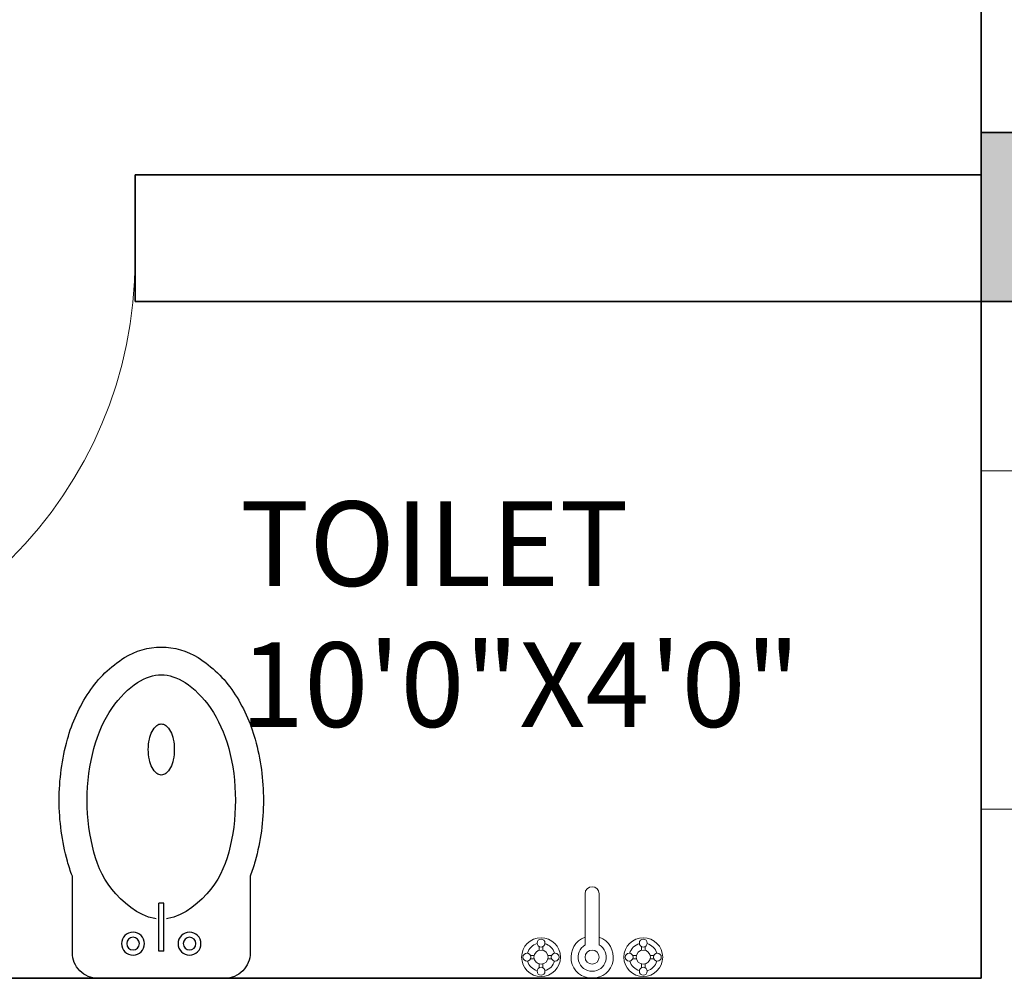
# Model space of a CAD drawing. Units: inches. Extents: x 3321 to 5237, y 11 to 1752.
# Tile 10 of 43: x 3724 to 3793, y 1377 to 1445. Entities that reach past the tile are written whole.
import ezdxf

# ---------------------------------------------------------------- set-up
doc = ezdxf.new("R2010")
doc.units = ezdxf.units.IN
for name, color, linetype, lineweight in [('A-ANNO-DIMS', 2, 'Continuous', 18), ('A-AREA-IDEN', 7, 'Continuous', 18), ('A-COLS', 1, 'Continuous', 35), ('A-DOOR', 4, 'Continuous', 18), ('A-GLAZ', 5, 'Continuous', 18), ('A-WALL', 7, 'Continuous', 35), ('Сантехника', 7, 'Continuous', 18)]:
    doc.layers.add(name, color=color, linetype=linetype, lineweight=lineweight)
doc.layers.add('SANTEH', color=7, linetype='Continuous')
doc.styles.get("Standard").update_dxf_attribs({"font": 'arial.ttf'})
doc.dimstyles.new('ISO-25', dxfattribs={"dimtxt": 9, "dimasz": 2.5, "dimexe": 1.25, "dimexo": 0.625, "dimtad": 1, "dimdec": 1, "dimlunit": 3, "dimtxsty": 'Standard', "dimcen": 2.5, "dimclrd": 4, "dimclre": 4, "dimclrt": 256, "dimadec": 0, "dimazin": 0, "dimtfac": 1, "dimtdec": 1, "dimtmove": 0, "dimatfit": 3, "dimfxl": 1, "dimarcsym": 0})

# ---------------------------------------------------------------- blocks, each defined once
blk = doc.blocks.new('*U5')
for p, q in [((0, 0), (0, -6)), ((-30, 0), (-30, -6))]:
    blk.add_line(p, q)
blk.add_lwpolyline([(0, 0), (0, 30), (-1.75, 30), (-1.75, 0)], close=True)
blk.add_arc((0, 0), 30, 90, 180)
blk = doc.blocks.new('K10-45')
at = {"layer": 'SANTEH'}
for p, q in [((-18.9, 83.4), (-18.9, 177.1)), ((-18.9, 177.1), (-8.9, 177.1)), ((-8.9, 83.4), (-8.9, 177.1)), ((-18.9, 83.4), (-8.9, 83.4))]:
    blk.add_line(p, q, dxfattribs=at)
for points in [[(160.3, 230.4, 0.023928), (169.9, 259.6, 0.067459), (186.1, 379, 0.067459), (169.9, 498.4, 0.079812), (127.5, 591.1, 0.107118), (58, 658.5, 0.139889), (-13.9, 679, 0.139889), (-85.8, 658.5, 0.107118), (-155.3, 591.1, 0.079812), (-197.7, 498.4, 0.067459), (-213.9, 379, 0.067459), (-197.7, 259.6, 0.023928), (-188.1, 230.4), (-188.1, 80.2, 0.414214), (-138.1, 30.2), (110.3, 30.2, 0.414214), (160.3, 80.2)], [(-39.4, 478.5, 0.052061), (-37.3, 458.3, 0.065919), (-32, 443.1, 0.104629), (-22.6, 431.5, 0.172287), (-13.9, 428.4, 0.172287), (-5.2, 431.5, 0.104629), (4.1, 443.1, 0.065919), (9.5, 458.3, 0.052061), (11.6, 478.5, 0.052061), (9.5, 498.7, 0.065919), (4.1, 513.9, 0.104629), (-5.2, 525.5, 0.172287), (-13.9, 528.6, 0.172287), (-22.6, 525.5, 0.104629), (-32, 513.9, 0.065919), (-37.3, 498.7, 0.052061)]]:
    blk.add_lwpolyline(points, format="xyb", close=True, dxfattribs=at)
blk.add_lwpolyline([(-3.9, 147), (-1.4, 147.2), (10.9, 150.3), (23, 155.1), (34.7, 161.4), (45.9, 168.8), (56.5, 177.2), (66.3, 186.2), (75.2, 195.5), (83.2, 205), (90.3, 214.7), (96.5, 224.5), (102, 234.5), (106.9, 244.7), (111.1, 255.3), (114.8, 266.2), (118.1, 277.6), (121.1, 289.3), (123.7, 301.4), (126, 313.8), (127.9, 326.5), (129.3, 339.5), (130.4, 352.6), (131.1, 365.8), (131.3, 379), (131.1, 392.2), (130.4, 405.4), (129.3, 418.5), (127.9, 431.4), (126, 444.2), (123.7, 456.6), (121.1, 468.7), (118.1, 480.4), (114.8, 491.7), (111.2, 502.6), (107.3, 513.1), (103, 523.1), (98.4, 532.7), (93.5, 541.9), (88.3, 550.7), (82.8, 559.1), (77.1, 567.1), (71, 574.6), (64.9, 581.7), (58.5, 588.3), (52.1, 594.4), (45.7, 600), (39.3, 605), (33, 609.4), (26.9, 613.2), (20.8, 616.4), (14.9, 619), (9, 621.1), (3.2, 622.7), (-2.5, 623.8), (-8.2, 624.5), (-13.9, 624.7), (-19.6, 624.5), (-25.3, 623.8), (-31, 622.7), (-36.8, 621.1), (-42.7, 619), (-48.6, 616.4), (-54.7, 613.2), (-60.9, 609.4), (-67.2, 605), (-73.5, 600), (-80, 594.4), (-86.4, 588.3), (-92.7, 581.7), (-98.9, 574.6), (-104.9, 567.1), (-110.6, 559.1), (-116.1, 550.7), (-121.3, 541.9), (-126.2, 532.7), (-130.8, 523.1), (-135.1, 513.1), (-139, 502.6), (-142.7, 491.7), (-146, 480.4), (-148.9, 468.7), (-151.5, 456.6), (-153.8, 444.2), (-155.7, 431.4), (-157.2, 418.5), (-158.2, 405.4), (-158.9, 392.2), (-159.1, 379), (-158.9, 365.8), (-158.2, 352.6), (-157.2, 339.5), (-155.7, 326.5), (-153.8, 313.8), (-151.5, 301.4), (-148.9, 289.3), (-146, 277.6), (-142.6, 266.2), (-138.9, 255.3), (-134.7, 244.7), (-129.8, 234.5), (-124.4, 224.5), (-118.1, 214.7), (-111, 205), (-103.1, 195.5), (-94.1, 186.2), (-84.3, 177.2), (-73.7, 168.8), (-62.5, 161.4), (-50.8, 155.1), (-38.7, 150.3), (-26.4, 147.2), (-23.9, 147)], dxfattribs=at)
for centre, radius in [((-69.2, 98.1), 22.4), ((41.4, 98.1), 22.4), ((-69.2, 98.1), 12.4), ((41.4, 98.1), 12.4)]:
    blk.add_circle(centre, radius, dxfattribs=at)
blk = doc.blocks.new('Faucet - Bathroom top')
for p, q in [((-3.75, 0.4788), (-3.75, 0.75)), ((-3.5, 0.482), (-3.5, 0.75)), ((3.5, 0.4788), (3.5, 0.75)), ((3.75, 0.482), (3.75, 0.75)), ((-4.107, 0.125), (-4.375, 0.125)), ((-3.1461, 0.125), (-2.875, 0.125)), ((3.143, 0.125), (2.875, 0.125)), ((4.1039, 0.125), (4.375, 0.125)), ((-4.1039, -0.125), (-4.375, -0.125)), ((-3.75, -0.4821), (-3.75, -0.75)), ((-3.5, -0.4789), (-3.5, -0.75)), ((-3.143, -0.125), (-2.875, -0.125)), ((3.1461, -0.125), (2.875, -0.125)), ((3.5, -0.4821), (3.5, -0.75)), ((3.75, -0.4789), (3.75, -0.75)), ((4.107, -0.125), (4.375, -0.125)), ((-0.5, -0.8639), (-0.5, -4.5)), ((0.5, -4.5), (0.5, -0.8631))]:
    blk.add_line(p, q)
for centre, radius in [((-3.625, 0), 1.375), ((-3.625, 1), 0.2795), ((3.625, 0), 1.375), ((3.625, 1), 0.2795), ((-4.625, 0), 0.2795), ((-3.625, 0), 0.5), ((-2.625, 0), 0.2795), ((0, 0), 0.5), ((2.625, 0), 0.2795), ((3.625, 0), 0.5), ((4.625, 0), 0.2795), ((-3.625, -1), 0.2795), ((3.625, -1), 0.2795)]:
    blk.add_circle(centre, radius)
for centre, radius, start, end in [((0, 0), 1.5, 289.6514, 250.3603), ((-3.625, 0), 1, 105.2407, 164.2093), ((-3.625, 0), 1, 16.44125, 74.07887), ((0, 0), 1, 300.3431, 239.7554), ((3.625, 0), 1, 106.12, 164.0884), ((3.625, 0), 1, 16.23422, 73.90469), ((-3.625, 0), 1, 196.2342, 253.9047), ((-3.625, 0), 1, 286.12, 344.0884), ((3.625, 0), 1, 196.4413, 254.0789), ((3.625, 0), 1, 285.2407, 344.2093), ((0, -4.5), 0.5, 180, 0)]:
    blk.add_arc(centre, radius, start, end)
blk = doc.blocks.new('COL-9X12-FURN-PLAN')
h = blk.add_hatch(color=256)
h.dxf.hatch_style = 1
h.paths.add_polyline_path([(0, 12), (0, 0), (9, 0), (9, 12)])
blk.add_lwpolyline([(0, 0), (9, 0), (9, 12), (0, 12)], close=True)
blk = doc.blocks.new('WIN-24IN-9IN-WALL')
for p, q in [((9, 24), (0, 24)), ((4, 24), (4, 0)), ((5, 24), (5, 0)), ((9, 0), (0, 0))]:
    blk.add_line(p, q)
blk = doc.blocks.new('*D192')
at = {"layer": 'A-ANNO-DIMS', "color": 4, "lineweight": -2, "transparency": 16777216}
for p, q in [((3704.375, 1473.484), (3704.375, 1457.036)), ((3791.689, 1473.484), (3791.689, 1457.036)), ((3706.875, 1458.286), (3789.189, 1458.286))]:
    blk.add_line(p, q, dxfattribs=at)
at = {"layer": 'A-ANNO-DIMS', "color": 4, "transparency": 16777216}
for points in [[(3706.875, 1458.702), (3706.875, 1457.869), (3704.375, 1458.286)], [(3789.189, 1458.702), (3789.189, 1457.869), (3791.689, 1458.286)]]:
    blk.add_solid(points, dxfattribs=at)
at = {"layer": 'Defpoints', "color": 0, "transparency": 16777216}
for p in [(3704.375, 1474.109), (3791.689, 1474.109), (3791.689, 1458.286)]:
    blk.add_point(p, dxfattribs=at)
at = {"layer": 'A-ANNO-DIMS', "transparency": 16777216, "insert": (3748.032, 1463.567), "char_height": 9, "attachment_point": 5}
blk.add_mtext('7\'-3 1/2" TYP.', dxfattribs=at)

msp = doc.modelspace()

# ---------------------------------------------------------------- linework, layer by layer
at = {"layer": 'A-WALL'}
for p, q in [((3791.689, 1626.339), (3791.689, 1434.339)), ((3731.689, 1434.339), (3791.689, 1434.339)), ((3731.689, 1425.339), (3731.689, 1434.339)), ((3731.689, 1425.339), (3791.689, 1425.339)), ((3791.689, 1425.339), (3791.689, 1377.339)), ((3671.689, 1377.339), (3791.689, 1377.339))]:
    msp.add_line(p, q, dxfattribs=at)

# ---------------------------------------------------------------- block references
at = {"layer": 'A-COLS'}
msp.add_blockref('COL-9X12-FURN-PLAN', (3791.689, 1425.339), dxfattribs=at)
at = {"layer": 'A-DOOR', "rotation": 180}
msp.add_blockref('*U5', (3701.689, 1428.339), dxfattribs=at)
at = {"layer": 'A-GLAZ'}
msp.add_blockref('WIN-24IN-9IN-WALL', (3791.689, 1389.339), dxfattribs=at)
at = {"layer": 'Сантехника', "xscale": -0.0362080263207385, "yscale": 0.0362080263207385, "zscale": 0.0362080263207385}
msp.add_blockref('K10-45', (3733.044, 1376.245), dxfattribs=at)
at = {"layer": 'Сантехника', "rotation": 180}
msp.add_blockref('Faucet - Bathroom top', (3764.1, 1378.839), dxfattribs=at)

# ---------------------------------------------------------------- texts
at = {"layer": 'A-AREA-IDEN', "insert": (3739.14, 1411.173), "char_height": 6, "attachment_point": 1}
msp.add_mtext_dynamic_manual_height_columns('TOILET\\P10\'0"X4\'0"', width=97.3114, gutter_width=25, heights=[0], dxfattribs=at)

# ---------------------------------------------------------------- dimensions: what is measured, and where the dimension line sits
at = {"layer": 'A-ANNO-DIMS'}
dim = msp.add_linear_dim(base=(3791.689, 1458.286), p1=(3704.375, 1474.109), p2=(3791.689, 1474.109), text='<> TYP.', dimstyle='ISO-25', override={"dimdec": 1, "dimlfac": 1, "dimrnd": 0, "dimzin": 1, "dimdsep": 46, "dimlunit": 4, "dimfrac": 2}, dxfattribs=at)
dim.commit()
dim.dimension.update_dxf_attribs({"geometry": '*D192', "text_midpoint": (3748.032, 1463.567)})

doc.saveas('drawing.dxf')
